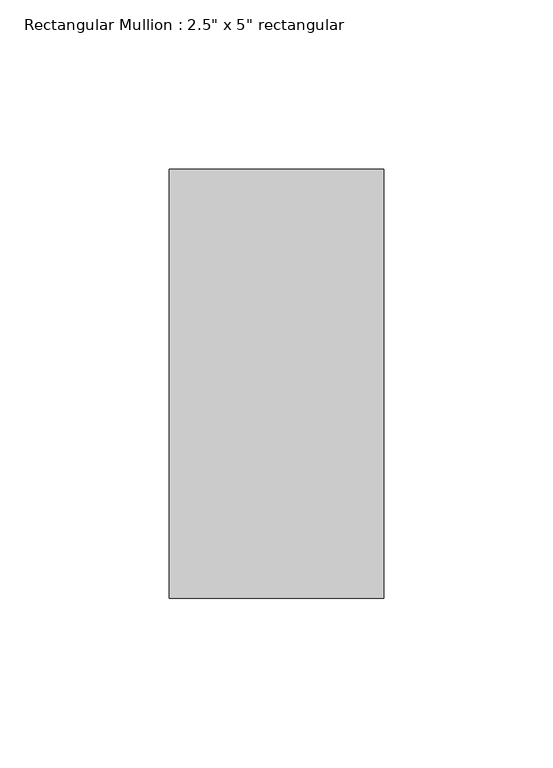
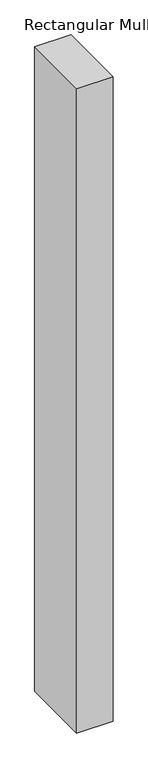
"""IFC4 building model written with IfcOpenShell, lengths in millimetres: member geometry."""

from ifc_helpers import new_model, si_unit, frame, origin, place, context, project, spatial, polyline, outline, extrude, source, transform, mapped, element, save


def member_34cc32ae(model_context):
    return source(origin(), model_context, "Body", "SweptSolid", [
        extrude(outline(polyline([(31.75, 63.5), (31.75, -63.5), (-31.75, -63.5), (-31.75, 63.5), (31.75, 63.5)])), frame((0.0, 0.0, -1187.4500002), z_axis=(0.0, 0.0, 1.0), x_axis=(1.0, 0.0, 0.0)), (0.0, 0.0, 1.0), 1187.4500002),
    ])


if __name__ == "__main__":
    model = new_model("IFC4")
    model_context = context("Model", 3, world=origin())
    ifc_project = project(units=[si_unit("LENGTHUNIT", "METRE", prefix="MILLI")], contexts=[model_context])
    site = spatial("IfcSite", under=ifc_project)
    building = spatial("IfcBuilding", under=site)
    placement = place(None, origin())
    member_shape = member_34cc32ae(model_context)
    element("IfcMember", 1, ObjectType="Rectangular Mullion : 2.5\" x 5\" rectangular", at=placement, inside=building, context=model_context, shape_type="MappedRepresentation", body=[
        mapped(member_shape, transform((0.0, 0.0, 0.0), x_axis=(1.0, 0.0, 0.0), y_axis=(0.0, 1.0, 0.0), z_axis=(0.0, 0.0, 1.0))),
    ])
    save(model, "model.ifc")

# Revit data of these elements
# Type "Rectangular Mullion : 2.5\" x 5\" rectangular"
#   built-in parameter 1007304 = 0.416667 (stored number, unit not read)
#   built-in parameter 1007301 = 0.104167 (stored number, unit not read)
#   built-in parameter 1007300 = 0.104167 (stored number, unit not read)
# Element 1 (IfcMember, "Rectangular Mullion : 2.5\" x 5\" rectangular")
#   Materials on its faces: "Aluminum"
# Materials
#   "Aluminum": class "Metal", colour RGB 247 247 247, transparency 0, Description = "Aluminum 6061", Cost = 0
